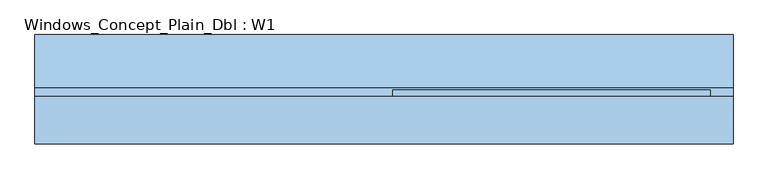
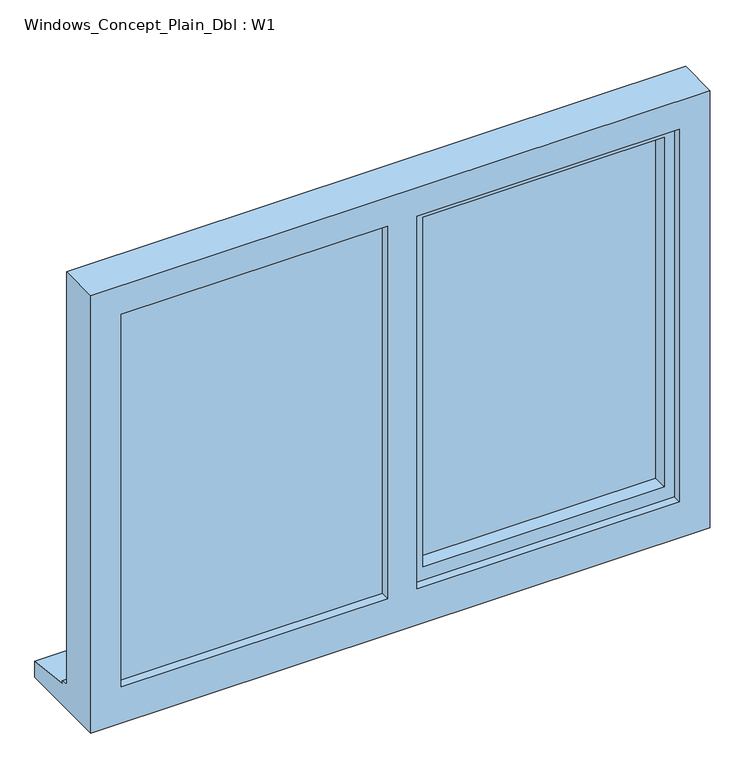
"""IFC4 building model written with IfcOpenShell, lengths in millimetres: window geometry, Windows_Concept_Plain_Dbl : W1."""

from ifc_helpers import new_model, si_unit, frame, origin, place, context, project, spatial, polyline, outline, extrude, faceted_brep, source, transform, mapped, element, save


def windows_concept_plain_dbl_w1_41c00efb(model_context):
    return source(origin(), model_context, "Body", "SolidModel", [
        faceted_brep([(-270.0, 22.9965678, 2070.0), (-270.0, 99.5435732, 2070.0), (-270.0, 99.5435732, 1263.0), (-270.0, 22.9965678, 1263.0), (-230.0, 51.9965678, 2030.0), (-230.0, 22.9965678, 2030.0), (-230.0, 22.9965678, 1303.0), (-230.0, 51.9965678, 1303.0), (-240.0, 75.9965678, 2040.0), (-240.0, 51.9965678, 2040.0), (-240.0, 51.9965678, 1293.0), (-240.0, 75.9965678, 1293.0), (-230.0, 99.5435732, 2030.0), (-230.0, 75.9965678, 2030.0), (-230.0, 75.9965678, 1303.0), (-230.0, 99.5435732, 1303.0), (284.6, 99.5435732, 1263.0), (284.6, 22.9965678, 1263.0), (244.6, 22.9965678, 1303.0), (244.6, 51.9965678, 1303.0), (254.6, 51.9965678, 1293.0), (254.6, 75.9965678, 1293.0), (244.6, 75.9965678, 1303.0), (244.6, 99.5435732, 1303.0), (284.6, 99.5435732, 2070.0), (284.6, 22.9965678, 2070.0), (244.6, 22.9965678, 2030.0), (244.6, 51.9965678, 2030.0), (254.6, 51.9965678, 2040.0), (254.6, 75.9965678, 2040.0), (244.6, 75.9965678, 2030.0), (244.6, 99.5435732, 2030.0)], [[[0, 1, 2, 3]], [[4, 5, 6, 7]], [[8, 9, 10, 11]], [[12, 13, 14, 15]], [[3, 2, 16, 17]], [[7, 6, 18, 19]], [[11, 10, 20, 21]], [[15, 14, 22, 23]], [[17, 16, 24, 25]], [[19, 18, 26, 27]], [[21, 20, 28, 29]], [[23, 22, 30, 31]], [[1, 24, 16, 2], [15, 23, 31, 12]], [[25, 24, 1, 0]], [[3, 17, 25, 0], [5, 26, 18, 6]], [[27, 26, 5, 4]], [[9, 28, 20, 10], [7, 19, 27, 4]], [[29, 28, 9, 8]], [[11, 21, 29, 8], [13, 30, 22, 14]], [[31, 30, 13, 12]]]),
        extrude(outline(polyline([(2050.0, -310.0), (2070.0, -310.0), (2070.0, -854.6), (1263.0, -854.6), (1263.0, -310.0), (1283.0, -310.0), (1283.0, -834.6), (2050.0, -834.6), (2050.0, -310.0)])), frame((0.0, 46.9965678, 0.0), z_axis=(0.0, 1.0, 0.0), x_axis=(0.0, 0.0, 1.0)), (0.0, 0.0, 1.0), 41.0),
        faceted_brep([(324.6, 4.9965678, 2110.0), (-894.6, 4.9965678, 2110.0), (-894.6, 4.9965678, 1200.0), (324.6, 4.9965678, 1200.0), (264.6, 4.9965678, 2050.0), (264.6, 4.9965678, 1275.0), (-252.0, 4.9965678, 1275.0), (-252.0, 4.9965678, 2050.0), (-310.0, 4.9965678, 2050.0), (-310.0, 4.9965678, 1275.0), (-834.6, 4.9965678, 1275.0), (-834.6, 4.9965678, 2050.0), (-894.6, 87.9965678, 2110.0), (-894.6, 87.9965678, 1251.0), (-894.6, 102.9965678, 1249.68767), (-894.6, 102.9965678, 1244.7449676), (-894.6, 195.9565678, 1233.8088847), (-894.6, 195.9565678, 1200.0), (324.6, 87.9965678, 2110.0), (324.6, 87.9965678, 1251.0), (-854.6, 87.9965678, 2070.0), (-854.6, 87.9965678, 1263.0), (-310.0, 87.9965678, 1263.0), (-310.0, 87.9965678, 2070.0), (-270.0, 87.9965678, 2070.0), (-270.0, 87.9965678, 1263.0), (284.6, 87.9965678, 1263.0), (284.6, 87.9965678, 2070.0), (-854.6, 22.9965678, 2070.0), (-854.6, 22.9965678, 1263.0), (-300.0, 22.9965678, 2070.0), (-300.0, 22.9965678, 1263.0), (-310.0, 22.9965678, 2050.0), (-834.6, 22.9965678, 2050.0), (-834.6, 22.9965678, 1275.0), (-310.0, 22.9965678, 1275.0), (-270.0, 22.9965678, 2070.0), (284.6, 22.9965678, 2070.0), (284.6, 22.9965678, 1263.0), (-270.0, 22.9965678, 1263.0), (264.6, 22.9965678, 2050.0), (-252.0, 22.9965678, 2050.0), (-252.0, 22.9965678, 1275.0), (264.6, 22.9965678, 1275.0), (-310.0, 46.9965678, 2070.0), (-300.0, 46.9965678, 2070.0), (324.6, 195.9565678, 1200.0), (324.6, 195.9565678, 1233.8088847), (324.6, 102.9965678, 1244.7449676), (324.6, 102.9965678, 1249.68767), (-300.0, 46.9965678, 1263.0), (-310.0, 46.9965678, 1263.0)], [[[0, 1, 2, 3], [4, 5, 6, 7], [8, 9, 10, 11]], [[2, 1, 12, 13, 14, 15, 16, 17]], [[13, 12, 18, 19], [20, 21, 22, 23], [24, 25, 26, 27]], [[21, 20, 28, 29]], [[28, 30, 31, 29], [32, 33, 34, 35]], [[36, 37, 38, 39], [40, 41, 42, 43]], [[33, 11, 10, 34]], [[1, 0, 18, 12]], [[28, 20, 23, 44, 45, 30]], [[27, 37, 36, 24]], [[11, 33, 32, 8]], [[40, 4, 7, 41]], [[19, 18, 0, 3, 46, 47, 48, 49]], [[27, 26, 38, 37]], [[4, 40, 43, 5]], [[45, 50, 31, 30]], [[50, 45, 44, 51]], [[51, 44, 23, 22]], [[25, 24, 36, 39]], [[41, 7, 6, 42]], [[8, 32, 35, 9]], [[46, 3, 2, 17]], [[47, 46, 17, 16]], [[48, 47, 16, 15]], [[49, 48, 15, 14]], [[19, 49, 14, 13]], [[22, 21, 29, 31, 50, 51]], [[26, 25, 39, 38]], [[6, 5, 43, 42]], [[35, 34, 10, 9]]]),
        extrude(outline(polyline([(-854.6, 46.9965678), (-300.0, 46.9965678), (-300.0, 22.9965678), (-854.6, 22.9965678), (-854.6, 46.9965678)])), frame((0.0, 0.0, 1263.0), z_axis=(0.0, 0.0, 1.0), x_axis=(1.0, 0.0, 0.0)), (0.0, 0.0, 1.0), 807.0),
        extrude(outline(polyline([(254.6, 51.9965678), (-240.0, 51.9965678), (-240.0, 75.9965678), (254.6, 75.9965678), (254.6, 51.9965678)])), frame((0.0, 0.0, 1293.0), z_axis=(0.0, 0.0, 1.0), x_axis=(1.0, 0.0, 0.0)), (0.0, 0.0, 1.0), 747.0),
    ])


if __name__ == "__main__":
    model = new_model("IFC4")
    model_context = context("Model", 3, world=origin())
    ifc_project = project(units=[si_unit("LENGTHUNIT", "METRE", prefix="MILLI")], contexts=[model_context])
    site = spatial("IfcSite", under=ifc_project)
    building = spatial("IfcBuilding", under=site)
    placement = place(None, origin())
    windows_concept_plain_dbl_w1_shape = windows_concept_plain_dbl_w1_41c00efb(model_context)
    element("IfcWindow", 1, ObjectType="Windows_Concept_Plain_Dbl : W1", at=placement, inside=building, context=model_context, shape_type="MappedRepresentation", body=[
        mapped(windows_concept_plain_dbl_w1_shape, transform((0.0, 0.0, 0.0), x_axis=(1.0, 0.0, 0.0), y_axis=(0.0, 1.0, 0.0), z_axis=(0.0, 0.0, 1.0))),
    ])
    save(model, "model.ifc")

# Revit data of these elements
# Type "Windows_Concept_Plain_Dbl : W1"
#   Type Mark = "56"
#   Operation = "DoublePanelVertical"
#   Construction Type Id = "GSP4R"
#   Manufacturer = "Revit"
#   Keynote = "L10"
#   Analytic Construction = "1/8 in Pilkington single glazing"
#   Visual Light Transmittance = 0.9
#   Solar Heat Gain Coefficient = 0.78
#   Rough Width = 1219.2 mm
#   Rough Height = 910 mm
#   Height = 910 mm
#   Width = 1219.2 mm
#   Heat Transfer Coefficient (U) = 3.6886 W/(m²·K)
#   FrameOffset - External = 50 mm
#   Default Head Height = 2110 mm
#   Vis - Cavity Closers = yes
#   Define Thermal Properties by = 1
#   Material Trim = Window Frame
#   Material Glass = Glass
#   Material Frame = Window Frame
#   Wall Closure = (empty or 0)
# Element 1 (IfcWindow, "Windows_Concept_Plain_Dbl : W1")
#   Materials on its faces: "Window Frame", "Glass"
# Materials
#   "Window Frame": colour RGB 249 249 249, transparency 0, Keynote = "L10", Cost = 0
#   "Glass": class "Glass", colour RGB 0 128 192, transparency 0.9, Description = "Soda Lime Glass", Cost = 0
